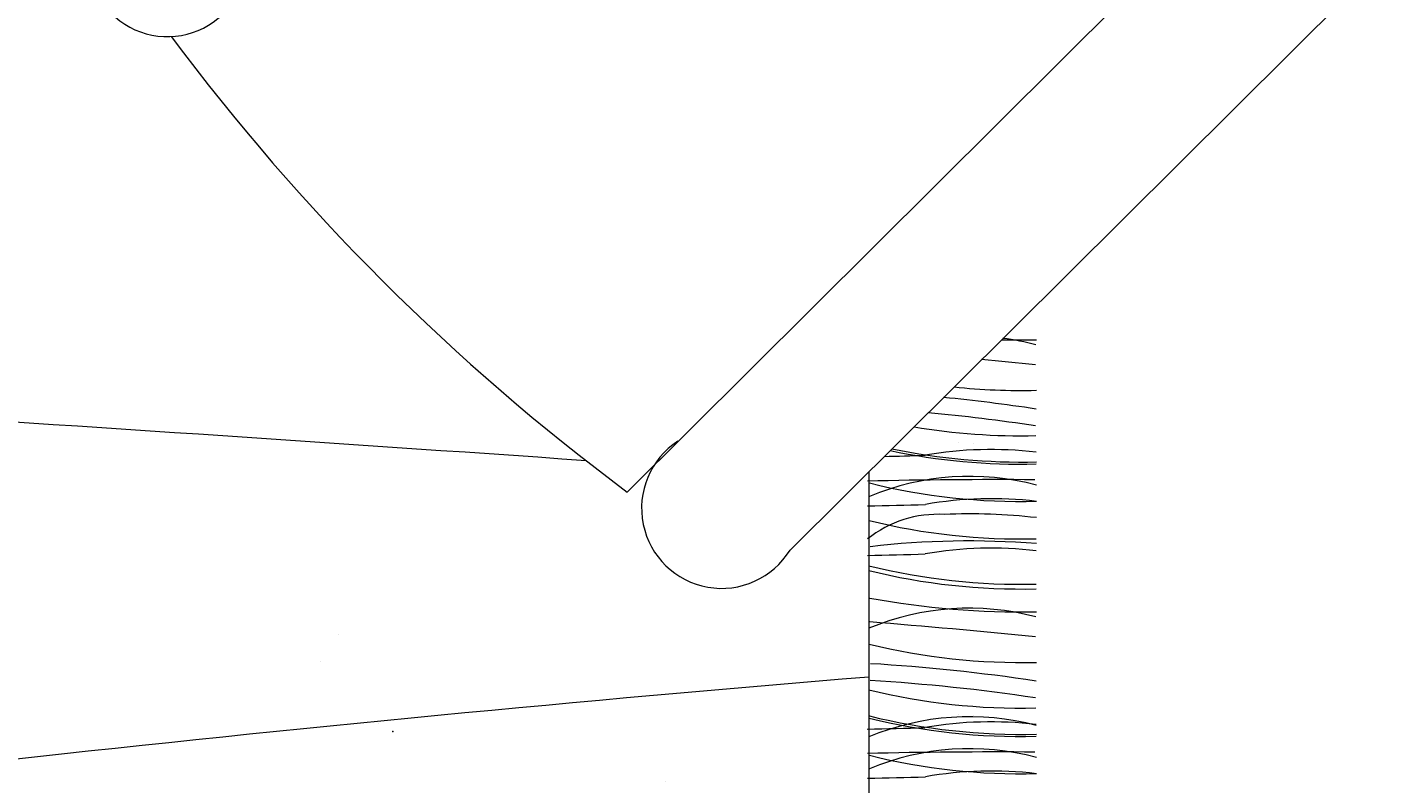
# Model space of a CAD drawing. Units: inches. Extents: x 182 to 1022, y -617 to 111.
# Tile 13 of 33: x 363 to 410, y -276 to -250. Entities that reach past the tile are written whole.
import ezdxf

# ---------------------------------------------------------------- set-up
doc = ezdxf.new("R2010")
doc.units = ezdxf.units.IN
doc.header["$MEASUREMENT"] = 0
doc.layers.add('A-ANNO-DIMS', color=2, linetype='Continuous', lineweight=18)
doc.layers.add('furniture', color=50, linetype='Continuous', lineweight=15, transparency=0.8)
doc.styles.get("Standard").update_dxf_attribs({"font": 'arial.ttf'})
doc.dimstyles.get("Standard").update_dxf_attribs({"dimtxt": 0.18, "dimasz": 0.18, "dimexe": 0.18, "dimexo": 0.0625, "dimgap": 0.09, "dimtad": 0, "dimtih": 1, "dimtoh": 1, "dimdec": 1, "dimzin": 0, "dimdsep": 46, "dimlunit": 4, "dimtxsty": 'Standard', "dimcen": 0.09, "dimadec": 0, "dimazin": 0, "dimtfac": 1, "dimtdec": 1, "dimtofl": 0, "dimtmove": 0, "dimatfit": 3, "dimfxl": 1, "dimtolj": 1, "dimtzin": 0, "dimarcsym": 0})

# ---------------------------------------------------------------- blocks, each defined once
blk = doc.blocks.new('LOUNGE-SEATING-GROUP')
for p, q in [((151.54, 48.98), (131.464, 29.017)), ((125.939, 30.989), (142.717, 47.686)), ((137.17, 32.684), (137.17, 32.684)), ((137.705, 32.64), (137.705, 32.64)), ((134.145, 31.682), (134.145, 5.694)), ((116.119, 26.161), (116.119, 26.161)), ((116.119, 26.161), (116.119, 26.161)), ((115.507, 25.236), (115.507, 25.236)), ((115.507, 25.236), (115.507, 25.236)), ((117.488, 23.122), (117.488, 23.122)), ((137.17, 23.434), (137.17, 23.434)), ((137.705, 23.39), (137.705, 23.39)), ((127.231, 21.162), (127.231, 21.162))]:
    blk.add_line(p, q)
for centre, radius, start, end in [((110.325, 49.163), 2.706, 123.6335, 326.3665), ((170.791, 91.372), 75.219, 216.66127, 233.39506), ((139.339, 64.774), 28.62, 268.619, 270.9805), ((137.55, 27.446), 8.837, 75.1387, 82.5478), ((114.367, -215.001), 251.596, 84.19829, 84.6171), ((139.318, 55.991), 21.554, 263.9229, 271.3669), ((-225.395, -5012.463), 5056.639, 86.03178, 86.330686), ((130.58, -27.106), 61.61, 81.37714, 84.31935), ((130.566, -27.679), 61.61, 81.37714, 84.79861), ((139.301, 54.452), 21.554, 260.3159, 271.3669), ((129.144, 30.436), 2.72, 123.0924, 328.5307), ((139.309, 53.489), 21.554, 258.0993, 271.3669), ((139.321, 53.561), 21.554, 258.2362, 271.3669), ((138.287, 19.638), 12.794, 83.1171, 100.0651), ((131.541, 174.878), 142.714, 271.25348, 271.81091), ((137.568, 22.685), 8.837, 75.1387, 112.6902), ((138.51, -153.111), 184.521, 89.60659, 91.37204), ((139.323, 52.222), 21.554, 256.1427, 271.3669), ((131.553, 173.209), 142.714, 271.02248, 271.81091), ((138.299, 17.969), 12.794, 83.1171, 100.0651), ((136.489, 26.377), 3.854, 86.8256, 128.3436), ((137.592, 10.303), 19.942, 83.5587, 92.5565), ((139.313, 50.947), 21.554, 256.1427, 271.3669), ((137.543, 0.21), 29.116, 85.4936, 96.6298), ((131.547, 171.527), 142.714, 271.02248, 271.81091), ((138.293, 16.287), 12.794, 83.1171, 100.0651), ((139.308, 49.408), 21.554, 256.1427, 271.3669), ((139.307, 49.248), 21.554, 256.1427, 271.3669), ((139.339, 55.534), 28.62, 259.5961, 270.9805), ((137.55, 18.206), 8.837, 75.1387, 112.6902), ((114.367, -224.24), 251.596, 84.19829, 85.48538), ((139.318, 46.751), 21.554, 256.1427, 271.3669), ((130.58, -36.346), 61.61, 81.37714, 86.63558), ((219.704, -1016.256), 1044.469, 94.698728, 96.310761), ((130.566, -36.919), 61.61, 81.37714, 86.63558), ((139.301, 45.202), 21.554, 256.1427, 271.3669), ((137.554, 14.519), 8.837, 75.1387, 112.6902), ((139.309, 44.239), 21.554, 256.1427, 271.3669), ((139.321, 44.311), 21.554, 256.1427, 271.3669), ((138.287, 10.388), 12.794, 83.1171, 100.0651), ((131.541, 165.628), 142.714, 271.02248, 271.81091), ((137.568, 13.435), 8.837, 75.1387, 112.6902), ((138.51, -162.361), 184.521, 89.60659, 91.37204), ((139.323, 42.972), 21.554, 256.1427, 271.3669), ((131.553, 163.959), 142.714, 271.02248, 271.81091), ((138.299, 8.719), 12.794, 83.1171, 100.0651)]:
    blk.add_arc(centre, radius, start, end)
blk.add_point((117.972, 22.852))
blk = doc.blocks.new('*D27')
at = {"layer": 'A-ANNO-DIMS', "color": 0, "lineweight": -2, "transparency": 16777216}
for p, q in [((409.45, -214.092), (432.299, -214.092)), ((432.119, -214.272), (432.119, -255.274)), ((432.119, -296.642), (432.119, -255.64)), ((409.45, -296.822), (432.299, -296.822))]:
    blk.add_line(p, q, dxfattribs=at)
at = {"layer": 'A-ANNO-DIMS', "color": 0, "transparency": 16777216}
for points in [[(432.089, -214.272), (432.149, -214.272), (432.119, -214.092)], [(432.089, -296.642), (432.149, -296.642), (432.119, -296.822)]]:
    blk.add_solid(points, dxfattribs=at)
at = {"layer": 'Defpoints', "color": 0, "transparency": 16777216}
for p in [(409.388, -214.092), (432.119, -214.092), (409.388, -296.822)]:
    blk.add_point(p, dxfattribs=at)
at = {"layer": 'A-ANNO-DIMS', "color": 0, "transparency": 16777216, "insert": (432.119, -255.457), "char_height": 0.18, "attachment_point": 5}
blk.add_mtext('\\A1;6\'-10 1/2" TYP.', dxfattribs=at)

msp = doc.modelspace()

# ---------------------------------------------------------------- block references
at = {"layer": 'furniture'}
msp.add_blockref('LOUNGE-SEATING-GROUP', (257.848, -296.822), dxfattribs=at)

# ---------------------------------------------------------------- dimensions: what is measured, and where the dimension line sits
at = {"layer": 'A-ANNO-DIMS'}
dim = msp.add_linear_dim(base=(432.119, -214.092), p1=(409.388, -296.822), p2=(409.388, -214.092), angle=90, text='<> TYP.', dimstyle='Standard', override={"dimdec": 1, "dimlfac": 1, "dimrnd": 0, "dimzin": 1, "dimdsep": 46, "dimlunit": 4, "dimfrac": 2}, dxfattribs=at)
dim.commit()
dim.dimension.update_dxf_attribs({"geometry": '*D27', "text_midpoint": (432.119, -255.457)})

doc.saveas('drawing.dxf')
